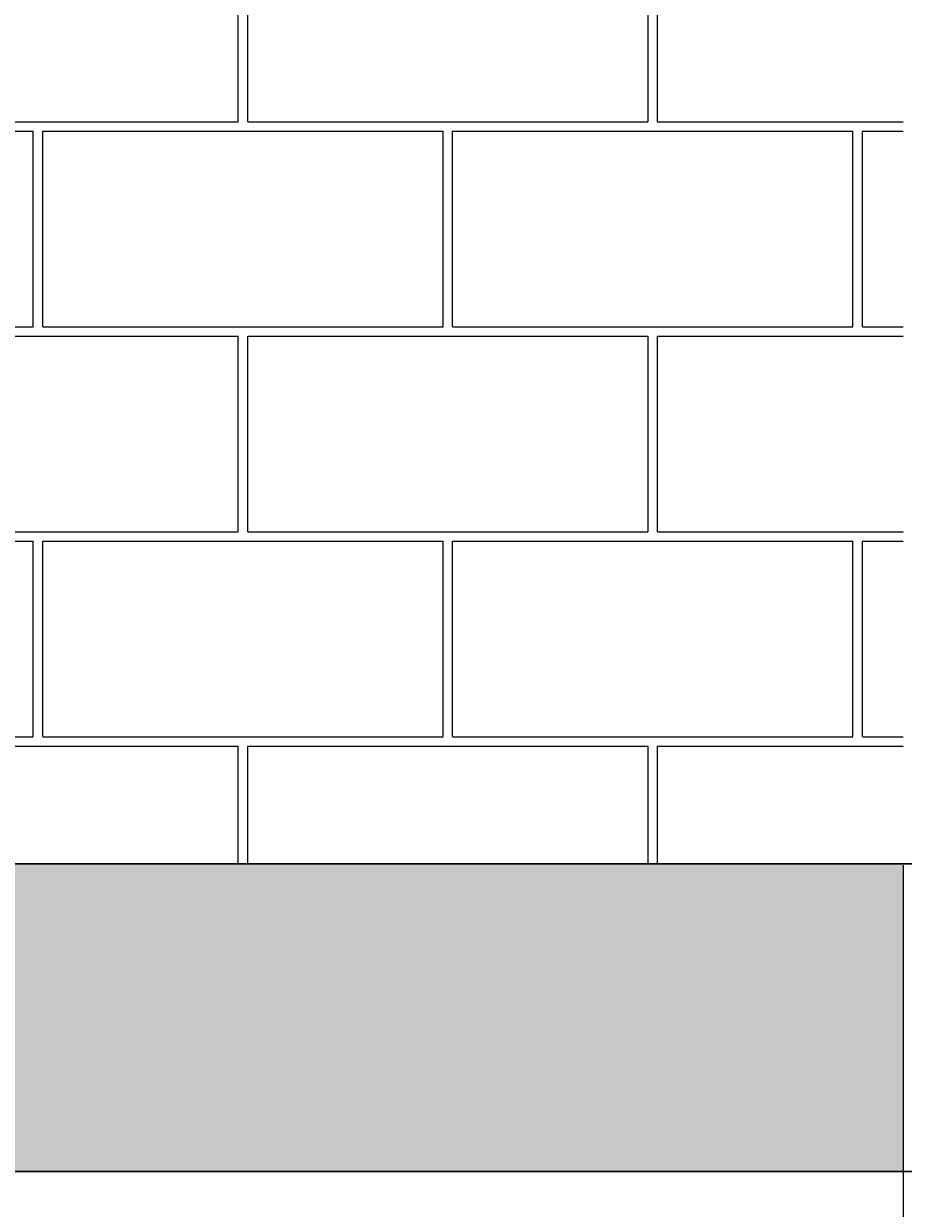
# Model space of a CAD drawing. Units: inches. Extents: x -301 to 715, y -607 to 364.
# Tile 133 of 141: x 362 to 413, y -510 to -440. Entities that reach past the tile are written whole.
import ezdxf

# ---------------------------------------------------------------- set-up
doc = ezdxf.new("R2010")
doc.units = ezdxf.units.IN
doc.header["$MEASUREMENT"] = 0
for name, color, linetype, lineweight in [('A-ANNO-DIMS', 2, 'Continuous', 18), ('A-ELEV', 220, 'Continuous', 30), ('A-ELEV-PATT', 4, 'Continuous', 13)]:
    doc.layers.add(name, color=color, linetype=linetype, lineweight=lineweight)
doc.styles.get("Standard").update_dxf_attribs({"font": 'arial.ttf'})
doc.dimstyles.get("Standard").update_dxf_attribs({"dimtxt": 0.18, "dimasz": 0.18, "dimexe": 0.18, "dimexo": 0.0625, "dimgap": 0.09, "dimtad": 0, "dimtih": 1, "dimtoh": 1, "dimdec": 1, "dimzin": 0, "dimdsep": 46, "dimlunit": 4, "dimtxsty": 'Standard', "dimcen": 0.09, "dimclrd": 3, "dimclre": 4, "dimclrt": 6, "dimadec": 0, "dimazin": 0, "dimtfac": 1, "dimtdec": 1, "dimtofl": 0, "dimtmove": 0, "dimatfit": 3, "dimfxl": 1, "dimtfill": 2, "dimtfillclr": 51, "dimtolj": 1, "dimtzin": 0, "dimarcsym": 0})

# ---------------------------------------------------------------- blocks, each defined once
blk = doc.blocks.new('*D196')
at = {"layer": 'A-ANNO-DIMS', "color": 4, "lineweight": -2, "transparency": 16777216}
for p, q in [((360.018, -441.615), (360.018, -606.789)), ((413.018, -489.615), (413.018, -606.789))]:
    blk.add_line(p, q, dxfattribs=at)
at = {"layer": 'A-ANNO-DIMS', "color": 3, "lineweight": -2, "transparency": 16777216}
for p, q in [((360.198, -606.609), (386.185, -606.609)), ((412.838, -606.609), (386.851, -606.609))]:
    blk.add_line(p, q, dxfattribs=at)
at = {"layer": 'A-ANNO-DIMS', "color": 3, "transparency": 16777216}
for points in [[(360.198, -606.579), (360.198, -606.639), (360.018, -606.609)], [(412.838, -606.579), (412.838, -606.639), (413.018, -606.609)]]:
    blk.add_solid(points, dxfattribs=at)
at = {"layer": 'Defpoints', "color": 0, "transparency": 16777216}
for p in [(360.018, -441.552), (413.018, -489.552), (413.018, -606.609)]:
    blk.add_point(p, dxfattribs=at)
at = {"layer": 'A-ANNO-DIMS', "color": 6, "transparency": 16777216, "insert": (386.518, -606.609), "char_height": 0.18, "attachment_point": 5, "bg_fill": 1, "box_fill_scale": 1.25, "bg_fill_color": 51, "bg_fill_transparency": 0}
blk.add_mtext('\\A1;4\'-5"', dxfattribs=at)
blk = doc.blocks.new('*D197')
at = {"layer": 'A-ANNO-DIMS', "color": 4, "lineweight": -2, "transparency": 16777216}
for p, q in [((413.018, -489.615), (413.018, -606.789)), ((461.018, -489.615), (461.018, -606.789))]:
    blk.add_line(p, q, dxfattribs=at)
at = {"layer": 'A-ANNO-DIMS', "color": 3, "lineweight": -2, "transparency": 16777216}
for p, q in [((413.198, -606.609), (436.685, -606.609)), ((460.838, -606.609), (437.351, -606.609))]:
    blk.add_line(p, q, dxfattribs=at)
at = {"layer": 'A-ANNO-DIMS', "color": 3, "transparency": 16777216}
for points in [[(413.198, -606.579), (413.198, -606.639), (413.018, -606.609)], [(460.838, -606.579), (460.838, -606.639), (461.018, -606.609)]]:
    blk.add_solid(points, dxfattribs=at)
at = {"layer": 'Defpoints', "color": 0, "transparency": 16777216}
for p in [(413.018, -489.552), (461.018, -489.552), (461.018, -606.609)]:
    blk.add_point(p, dxfattribs=at)
at = {"layer": 'A-ANNO-DIMS', "color": 6, "transparency": 16777216, "insert": (437.018, -606.609), "char_height": 0.18, "attachment_point": 5, "bg_fill": 1, "box_fill_scale": 1.25, "bg_fill_color": 51, "bg_fill_transparency": 0}
blk.add_mtext('\\A1;4\'-0"', dxfattribs=at)
blk = doc.blocks.new('*D200')
at = {"layer": 'A-ANNO-DIMS', "color": 4, "lineweight": -2, "transparency": 16777216}
for p, q in [((412.955, -393.552), (121.926, -393.552)), ((412.955, -489.552), (121.926, -489.552))]:
    blk.add_line(p, q, dxfattribs=at)
at = {"layer": 'A-ANNO-DIMS', "color": 3, "lineweight": -2, "transparency": 16777216}
for p, q in [((122.106, -393.732), (122.106, -441.371)), ((122.106, -489.372), (122.106, -441.734))]:
    blk.add_line(p, q, dxfattribs=at)
at = {"layer": 'A-ANNO-DIMS', "color": 3, "transparency": 16777216}
for points in [[(122.076, -393.732), (122.136, -393.732), (122.106, -393.552)], [(122.076, -489.372), (122.136, -489.372), (122.106, -489.552)]]:
    blk.add_solid(points, dxfattribs=at)
at = {"layer": 'Defpoints', "color": 0, "transparency": 16777216}
for p in [(122.106, -393.552), (413.018, -393.552), (413.018, -489.552)]:
    blk.add_point(p, dxfattribs=at)
at = {"layer": 'A-ANNO-DIMS', "color": 6, "transparency": 16777216, "insert": (122.106, -441.552), "char_height": 0.18, "attachment_point": 5, "bg_fill": 1, "box_fill_scale": 1.25, "bg_fill_color": 51, "bg_fill_transparency": 0}
blk.add_mtext('\\A1;8\'-0"', dxfattribs=at)

msp = doc.modelspace()

# ---------------------------------------------------------------- hatches: boundary and pattern name
at = {"layer": 'A-ELEV-PATT'}
h = msp.add_hatch(dxfattribs=at)
h.set_pattern_fill('AR-B816C', color=256, scale=1.5)
h.set_pattern_definition([(0, (458.621, 9.325), (12, 12), [23.4375, -0.5625]), (0, (446.621, 9.887), (12, 12), [23.4375, -0.5625]), (90, (458.621, 9.325), (-12, 12), [-12.5625, 11.4375]), (90, (458.059, 9.325), (-12, 12), [-12.5625, 11.4375])])
h.paths.add_polyline_path([(254.018, -489.552), (413.018, -489.552), (413.018, -393.552), (461.018, -393.552), (461.018, -489.552), (591.518, -489.552), (591.518, -369.552), (254.018, -369.552)])
h.paths.add_polyline_path([(310.018, -393.552), (360.018, -393.552), (360.018, -441.552), (310.018, -441.552)], flags=16)
h.paths.add_polyline_path([(315.018, -398.552), (355.018, -398.552), (355.018, -436.552), (315.018, -436.552)], flags=0)
h.paths.add_polyline_path([(496.768, -393.552), (546.768, -393.552), (546.768, -441.552), (496.768, -441.552)], flags=16)
h.paths.add_polyline_path([(501.768, -398.552), (541.768, -398.552), (541.768, -436.552), (501.768, -436.552)], flags=0)
h = msp.add_hatch(dxfattribs=at)
h.set_pattern_fill('AR-CONC', color=256, scale=2)
h.set_pattern_definition([(50, (458.621, 9.325), (14.3452, -1.25504), [1.5, -16.5]), (355, (458.621, 9.325), (-2.77503, 15.04384), [1.2, -13.2]), (100.4514, (459.817, 9.22), (11.57018, 13.7888), [1.2748, -14.02284]), (46.1842, (458.621, 13.325), (21.3448, -3.3104), [2.25, -24.75]), (96.6356, (460.4, 13.049), (18.69324, 19.4824), [1.9122, -21.0343]), (351.184, (458.62, 13.325), (18.6932, 19.4824), [1.8, -19.8]), (21, (460.621, 12.325), (11.93814, -8.05238), [1.5, -16.5]), (326, (460.621, 12.325), (4.8663, 14.503), [1.2, -13.2]), (71.4514, (461.616, 11.654), (16.80445, 6.45062), [1.2748, -14.02284]), (37.5, (458.621, 9.325), (0.243197, 6.657877), [0, -13.04, 0, -13.4, 0, -13.25]), (7.5, (458.621, 9.325), (5.26139, 7.88823), [0, -7.64, 0, -12.74, 0, -5.05]), (327.5, (454.161, 9.325), (10.67645, -0.4511), [0, -5, 0, -15.6, 0, -20.7]), (317.5, (452.161, 9.325), (11.66372, 2.0021), [0, -6.5, 0, -10.36, 0, -14.7])])
h.paths.add_polyline_path([(254.018, -489.552), (254.018, -507.552), (413.018, -507.552), (413.018, -489.552)])
h.paths.add_polyline_path([(591.518, -507.552), (591.518, -489.552), (461.018, -489.552), (461.018, -507.552)])

# ---------------------------------------------------------------- linework, layer by layer
at = {"layer": 'A-ELEV'}
for p, q in [((254.018, -489.552), (591.518, -489.552)), ((254.018, -507.552), (591.518, -507.552))]:
    msp.add_line(p, q, dxfattribs=at)
for points in [[(254.018, -369.552), (591.518, -369.552), (591.518, -489.552), (254.018, -489.552)], [(254.018, -489.552), (591.518, -489.552), (591.518, -507.552), (254.018, -507.552)]]:
    msp.add_lwpolyline(points, close=True, dxfattribs=at)

# ---------------------------------------------------------------- dimensions: what is measured, and where the dimension line sits
at = {"layer": 'A-ANNO-DIMS'}
dim = msp.add_linear_dim(base=(122.106, -393.552), p1=(413.018, -489.552), p2=(413.018, -393.552), angle=90, dimstyle='Standard', override={"dimdec": 1, "dimlfac": 1, "dimrnd": 0, "dimzin": 1, "dimdsep": 46, "dimlunit": 4, "dimfrac": 2}, dxfattribs=at)
dim.commit()
dim.dimension.update_dxf_attribs({"geometry": '*D200', "text_midpoint": (122.106, -441.552)})
for base, p1, p2, picture, middle in [((413.018, -606.609), (360.018, -441.552), (413.018, -489.552), '*D196', (386.518, -606.609)), ((461.018, -606.609), (413.018, -489.552), (461.018, -489.552), '*D197', (437.018, -606.609))]:
    dim = msp.add_linear_dim(base=base, p1=p1, p2=p2, dimstyle='Standard', override={"dimdec": 1, "dimlfac": 1, "dimrnd": 0, "dimzin": 1, "dimdsep": 46, "dimlunit": 4, "dimfrac": 2}, dxfattribs=at)
    dim.commit()
    dim.dimension.update_dxf_attribs({"geometry": picture, "text_midpoint": middle})

doc.saveas('drawing.dxf')
